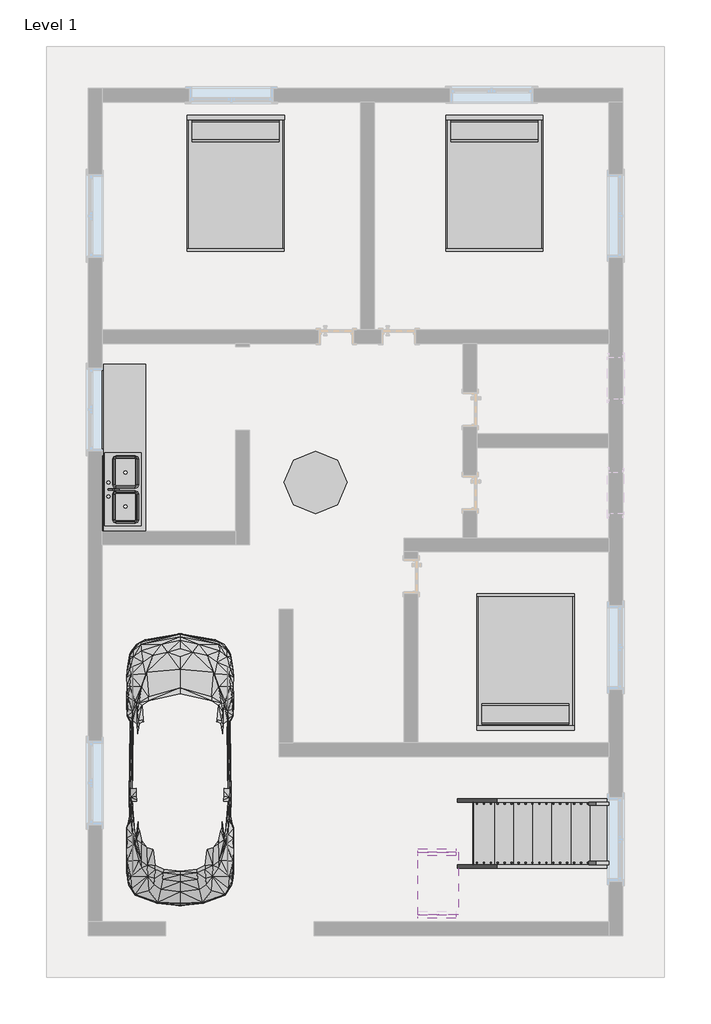
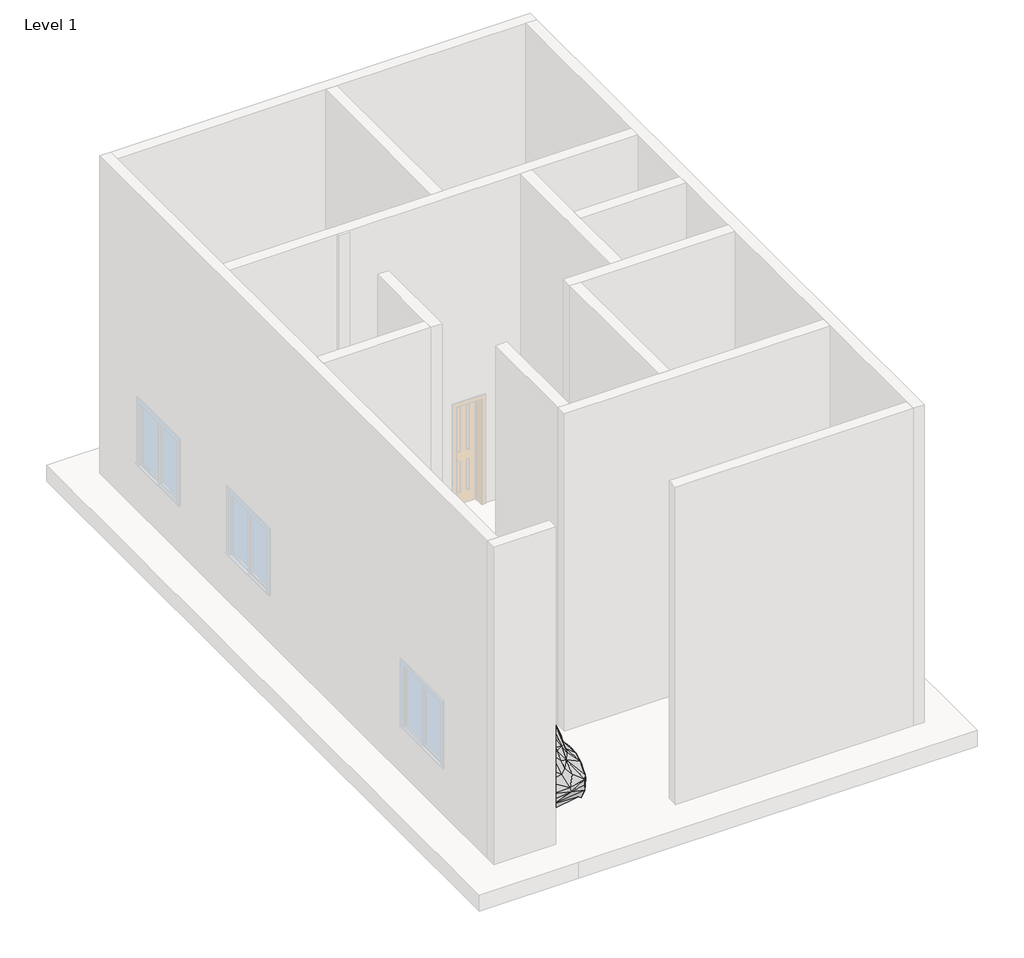
# One storey, part 2 of 2: 5 furniture elements, 4 members, 3 railings, 2 stair flights, 1 flow terminal, 1 proxy.
"""IFC4 building model written with IfcOpenShell, lengths in millimetres."""

from ifc_helpers import new_model, si_unit, frame, origin, place, context, project, spatial, polyline, outline, extrude, transform, mapped, element, save
from components import rpc_beetle_rpc_beetle_3ce7ba48, flow_terminal_a53be723, furniture_096e7f55, furniture_91b07d4a, furniture_905aceb5, stair_flight_75b00a3b, stair_flight_c315cc2a

model = new_model("IFC4")

# Units and contexts
model_context = context("Model", 3, world=origin())
ifc_project = project(units=[si_unit("LENGTHUNIT", "METRE", prefix="MILLI")], contexts=[model_context])

# Site, building, storey
site = spatial("IfcSite", under=ifc_project)
building = spatial("IfcBuilding", under=site)
storey = spatial("IfcBuildingStorey", under=building, Name="Level 1", Elevation=0.0)

# Proxy
placement = place(None, origin())
rpc_beetle_rpc_beetle_shape = rpc_beetle_rpc_beetle_3ce7ba48(model_context)
element("IfcBuildingElementProxy", 1, Name="RPC Beetle : RPC Beetle", ObjectType="RPC Beetle : RPC Beetle", at=placement, inside=storey, context=model_context, shape_type="MappedRepresentation", body=[
    mapped(rpc_beetle_rpc_beetle_shape, transform((-13294.6836698, -717.7093225, 0.0), x_axis=(1.0, 0.0, 0.0), y_axis=(0.0, 1.0, 0.0), z_axis=(0.0, 0.0, 1.0))),
])

# Flow terminal
flow_terminal_shape = flow_terminal_a53be723(model_context)
element("IfcFlowTerminal", 2, ObjectType="Sink Kitchen-Double : 42\" x 21\"", at=placement, inside=storey, context=model_context, shape_type="MappedRepresentation", body=[
    mapped(flow_terminal_shape, transform((-14130.5382687, 4600.601437, 0.0), x_axis=(0.0, 1.0, 0.0), y_axis=(-1.0, 0.0, 0.0), z_axis=(0.0, 0.0, 1.0))),
])

# Furniture
furniture_shape = furniture_096e7f55(model_context)
element("IfcFurniture", 3, ObjectType="Bed-Shaker : Double 56\" x 78\"", at=placement, inside=storey, context=model_context, shape_type="MappedRepresentation", body=[
    mapped(furniture_shape, transform((-12462.8336698, 10077.2906775, 0.0), x_axis=(1.0, 0.0, 0.0), y_axis=(0.0, 1.0, 0.0), z_axis=(0.0, 0.0, 1.0))),
])
element("IfcFurniture", 4, ObjectType="Bed-Shaker : Double 56\" x 78\"", at=placement, inside=storey, context=model_context, shape_type="MappedRepresentation", body=[
    mapped(furniture_shape, transform((-8678.2336698, 10077.2906775, 0.0), x_axis=(1.0, 0.0, 0.0), y_axis=(0.0, 1.0, 0.0), z_axis=(0.0, 0.0, 1.0))),
])
element("IfcFurniture", 5, ObjectType="Bed-Shaker : Double 56\" x 78\"", at=placement, inside=storey, context=model_context, shape_type="MappedRepresentation", body=[
    mapped(furniture_shape, transform((-8259.1336698, 1111.0906775, 0.0), x_axis=(-1.0, 0.0, 0.0), y_axis=(0.0, -1.0, 0.0), z_axis=(0.0, 0.0, 1.0))),
])
furniture_2_shape = furniture_91b07d4a(model_context)
element("IfcFurniture", 6, ObjectType="Counter Top w Sink : 24\" Depth", at=placement, inside=storey, context=model_context, shape_type="MappedRepresentation", body=[
    mapped(furniture_2_shape, transform((-14437.6836698, 5207.1529726, 0.0), x_axis=(0.0, 1.0, 0.0), y_axis=(-1.0, 0.0, 0.0), z_axis=(0.0, 0.0, 1.0))),
])
furniture_3_shape = furniture_905aceb5(model_context)
element("IfcFurniture", 7, ObjectType="Table-Dining Round w Chairs : 36\" Diameter", at=placement, inside=storey, context=model_context, shape_type="MappedRepresentation", body=[
    mapped(furniture_3_shape, transform((-11417.165637, 4902.769366, 0.0), x_axis=(1.0, 0.0, 0.0), y_axis=(0.0, 1.0, 0.0), z_axis=(0.0, 0.0, 1.0))),
])

# Members
element("IfcMember", 8, ObjectType="Stringer - 2\" Width", at=placement, inside=storey, context=model_context, shape_type="SweptSolid", body=[
    extrude(outline(polyline([(0.0, -7020.8836698), (212.114512, -7020.8836698), (2074.7811786, -10094.2836698), (1718.3724171, -10094.2836698), (0.0, -7258.9691815), (0.0, -7020.8836698)])), frame((0.0, -920.9093225, 0.0), z_axis=(0.0, 1.0, 0.0), x_axis=(0.0, 0.0, 1.0)), (0.0, 0.0, 1.0), 50.8),
])
element("IfcMember", 9, ObjectType="Stringer - 2\" Width", at=placement, inside=storey, context=model_context, shape_type="SweptSolid", body=[
    extrude(outline(polyline([(0.0, -7020.8836698), (212.114512, -7020.8836698), (2074.7811786, -10094.2836698), (1718.3724171, -10094.2836698), (0.0, -7258.9691815), (0.0, -7020.8836698)])), frame((0.0, 44.2906775, 0.0), z_axis=(0.0, 1.0, 0.0), x_axis=(0.0, 0.0, 1.0)), (0.0, 0.0, 1.0), 50.8),
])
element("IfcMember", 10, ObjectType="Stringer - 2\" Width", at=placement, inside=storey, context=model_context, shape_type="SweptSolid", body=[
    extrude(outline(polyline([(2244.114512, -9814.8836698), (1887.7057504, -9814.8836698), (2226.3724171, -9256.0836698), (2582.7811786, -9256.0836698), (2244.114512, -9814.8836698)])), frame((0.0, -692.3093225, 0.0), z_axis=(0.0, 1.0, 0.0), x_axis=(0.0, 0.0, 1.0)), (0.0, 0.0, 1.0), 50.8),
])
element("IfcMember", 11, ObjectType="Stringer - 2\" Width", at=placement, inside=storey, context=model_context, shape_type="SweptSolid", body=[
    extrude(outline(polyline([(2244.114512, -9814.8836698), (1887.7057504, -9814.8836698), (2226.3724171, -9256.0836698), (2582.7811786, -9256.0836698), (2244.114512, -9814.8836698)])), frame((0.0, -1657.5093225, 0.0), z_axis=(0.0, 1.0, 0.0), x_axis=(0.0, 0.0, 1.0)), (0.0, 0.0, 1.0), 50.8),
])

# Railings
element("IfcRailing", 12, ObjectType="Handrail - Rectangular", at=placement, inside=storey, context=model_context, shape_type="SweptSolid", body=[
    extrude(outline(polyline([(1024.3318731, -7020.8836698), (1083.7333333, -7020.8836698), (2946.4, -10094.2836698), (2886.9985397, -10094.2836698), (1024.3318731, -7020.8836698)])), frame((0.0, -6.5093225, 0.0), z_axis=(0.0, 1.0, 0.0), x_axis=(0.0, 0.0, 1.0)), (0.0, 0.0, 1.0), 50.8),
    extrude(outline(polyline([(2865.8318731, -10059.3586698), (2877.3773276, -10078.4086698), (1862.6666667, -10078.4086698), (1862.6666667, -10059.3586698), (2865.8318731, -10059.3586698)])), frame((0.0, 9.3656775, 0.0), z_axis=(0.0, 1.0, 0.0), x_axis=(0.0, 0.0, 1.0)), (0.0, 0.0, 1.0), 19.05),
    extrude(outline(polyline([(2804.2561155, -9957.7586698), (2815.80157, -9976.8086698), (1862.6666667, -9976.8086698), (1862.6666667, -9957.7586698), (2804.2561155, -9957.7586698)])), frame((0.0, 9.3656775, 0.0), z_axis=(0.0, 1.0, 0.0), x_axis=(0.0, 0.0, 1.0)), (0.0, 0.0, 1.0), 19.05),
    extrude(outline(polyline([(2742.6803579, -9856.1586698), (2754.2258125, -9875.2086698), (1862.6666667, -9875.2086698), (1862.6666667, -9856.1586698), (2742.6803579, -9856.1586698)])), frame((0.0, 9.3656775, 0.0), z_axis=(0.0, 1.0, 0.0), x_axis=(0.0, 0.0, 1.0)), (0.0, 0.0, 1.0), 19.05),
    extrude(outline(polyline([(2681.1046004, -9754.5586698), (2692.6500549, -9773.6086698), (1693.3333333, -9773.6086698), (1693.3333333, -9754.5586698), (2681.1046004, -9754.5586698)])), frame((0.0, 9.3656775, 0.0), z_axis=(0.0, 1.0, 0.0), x_axis=(0.0, 0.0, 1.0)), (0.0, 0.0, 1.0), 19.05),
    extrude(outline(polyline([(2619.5288428, -9652.9586698), (2631.0742973, -9672.0086698), (1693.3333333, -9672.0086698), (1693.3333333, -9652.9586698), (2619.5288428, -9652.9586698)])), frame((0.0, 9.3656775, 0.0), z_axis=(0.0, 1.0, 0.0), x_axis=(0.0, 0.0, 1.0)), (0.0, 0.0, 1.0), 19.05),
    extrude(outline(polyline([(2557.9530852, -9551.3586698), (2569.4985397, -9570.4086698), (1693.3333333, -9570.4086698), (1693.3333333, -9551.3586698), (2557.9530852, -9551.3586698)])), frame((0.0, 9.3656775, 0.0), z_axis=(0.0, 1.0, 0.0), x_axis=(0.0, 0.0, 1.0)), (0.0, 0.0, 1.0), 19.05),
    extrude(outline(polyline([(2496.3773276, -9449.7586698), (2507.9227822, -9468.8086698), (1524.0, -9468.8086698), (1524.0, -9449.7586698), (2496.3773276, -9449.7586698)])), frame((0.0, 9.3656775, 0.0), z_axis=(0.0, 1.0, 0.0), x_axis=(0.0, 0.0, 1.0)), (0.0, 0.0, 1.0), 19.05),
    extrude(outline(polyline([(2434.80157, -9348.1586698), (2446.3470246, -9367.2086698), (1524.0, -9367.2086698), (1524.0, -9348.1586698), (2434.80157, -9348.1586698)])), frame((0.0, 9.3656775, 0.0), z_axis=(0.0, 1.0, 0.0), x_axis=(0.0, 0.0, 1.0)), (0.0, 0.0, 1.0), 19.05),
    extrude(outline(polyline([(2373.2258125, -9246.5586698), (2384.771267, -9265.6086698), (1524.0, -9265.6086698), (1524.0, -9246.5586698), (2373.2258125, -9246.5586698)])), frame((0.0, 9.3656775, 0.0), z_axis=(0.0, 1.0, 0.0), x_axis=(0.0, 0.0, 1.0)), (0.0, 0.0, 1.0), 19.05),
    extrude(outline(polyline([(2311.6500549, -9144.9586698), (2323.1955094, -9164.0086698), (1354.6666667, -9164.0086698), (1354.6666667, -9144.9586698), (2311.6500549, -9144.9586698)])), frame((0.0, 9.3656775, 0.0), z_axis=(0.0, 1.0, 0.0), x_axis=(0.0, 0.0, 1.0)), (0.0, 0.0, 1.0), 19.05),
    extrude(outline(polyline([(2250.0742973, -9043.3586698), (2261.6197519, -9062.4086698), (1354.6666667, -9062.4086698), (1354.6666667, -9043.3586698), (2250.0742973, -9043.3586698)])), frame((0.0, 9.3656775, 0.0), z_axis=(0.0, 1.0, 0.0), x_axis=(0.0, 0.0, 1.0)), (0.0, 0.0, 1.0), 19.05),
    extrude(outline(polyline([(2188.4985397, -8941.7586698), (2200.0439943, -8960.8086698), (1185.3333333, -8960.8086698), (1185.3333333, -8941.7586698), (2188.4985397, -8941.7586698)])), frame((0.0, 9.3656775, 0.0), z_axis=(0.0, 1.0, 0.0), x_axis=(0.0, 0.0, 1.0)), (0.0, 0.0, 1.0), 19.05),
    extrude(outline(polyline([(2126.9227822, -8840.1586698), (2138.4682367, -8859.2086698), (1185.3333333, -8859.2086698), (1185.3333333, -8840.1586698), (2126.9227822, -8840.1586698)])), frame((0.0, 9.3656775, 0.0), z_axis=(0.0, 1.0, 0.0), x_axis=(0.0, 0.0, 1.0)), (0.0, 0.0, 1.0), 19.05),
    extrude(outline(polyline([(2065.3470246, -8738.5586698), (2076.8924791, -8757.6086698), (1185.3333333, -8757.6086698), (1185.3333333, -8738.5586698), (2065.3470246, -8738.5586698)])), frame((0.0, 9.3656775, 0.0), z_axis=(0.0, 1.0, 0.0), x_axis=(0.0, 0.0, 1.0)), (0.0, 0.0, 1.0), 19.05),
    extrude(outline(polyline([(2003.771267, -8636.9586698), (2015.3167216, -8656.0086698), (1016.0, -8656.0086698), (1016.0, -8636.9586698), (2003.771267, -8636.9586698)])), frame((0.0, 9.3656775, 0.0), z_axis=(0.0, 1.0, 0.0), x_axis=(0.0, 0.0, 1.0)), (0.0, 0.0, 1.0), 19.05),
    extrude(outline(polyline([(1942.1955094, -8535.3586698), (1953.740964, -8554.4086698), (1016.0, -8554.4086698), (1016.0, -8535.3586698), (1942.1955094, -8535.3586698)])), frame((0.0, 9.3656775, 0.0), z_axis=(0.0, 1.0, 0.0), x_axis=(0.0, 0.0, 1.0)), (0.0, 0.0, 1.0), 19.05),
    extrude(outline(polyline([(1880.6197519, -8433.7586698), (1892.1652064, -8452.8086698), (1016.0, -8452.8086698), (1016.0, -8433.7586698), (1880.6197519, -8433.7586698)])), frame((0.0, 9.3656775, 0.0), z_axis=(0.0, 1.0, 0.0), x_axis=(0.0, 0.0, 1.0)), (0.0, 0.0, 1.0), 19.05),
    extrude(outline(polyline([(1819.0439943, -8332.1586698), (1830.5894488, -8351.2086698), (846.6666667, -8351.2086698), (846.6666667, -8332.1586698), (1819.0439943, -8332.1586698)])), frame((0.0, 9.3656775, 0.0), z_axis=(0.0, 1.0, 0.0), x_axis=(0.0, 0.0, 1.0)), (0.0, 0.0, 1.0), 19.05),
    extrude(outline(polyline([(1757.4682367, -8230.5586698), (1769.0136913, -8249.6086698), (846.6666667, -8249.6086698), (846.6666667, -8230.5586698), (1757.4682367, -8230.5586698)])), frame((0.0, 9.3656775, 0.0), z_axis=(0.0, 1.0, 0.0), x_axis=(0.0, 0.0, 1.0)), (0.0, 0.0, 1.0), 19.05),
    extrude(outline(polyline([(1695.8924791, -8128.9586698), (1707.4379337, -8148.0086698), (846.6666667, -8148.0086698), (846.6666667, -8128.9586698), (1695.8924791, -8128.9586698)])), frame((0.0, 9.3656775, 0.0), z_axis=(0.0, 1.0, 0.0), x_axis=(0.0, 0.0, 1.0)), (0.0, 0.0, 1.0), 19.05),
    extrude(outline(polyline([(1634.3167216, -8027.3586698), (1645.8621761, -8046.4086698), (677.3333333, -8046.4086698), (677.3333333, -8027.3586698), (1634.3167216, -8027.3586698)])), frame((0.0, 9.3656775, 0.0), z_axis=(0.0, 1.0, 0.0), x_axis=(0.0, 0.0, 1.0)), (0.0, 0.0, 1.0), 19.05),
    extrude(outline(polyline([(1572.740964, -7925.7586698), (1584.2864185, -7944.8086698), (677.3333333, -7944.8086698), (677.3333333, -7925.7586698), (1572.740964, -7925.7586698)])), frame((0.0, 9.3656775, 0.0), z_axis=(0.0, 1.0, 0.0), x_axis=(0.0, 0.0, 1.0)), (0.0, 0.0, 1.0), 19.05),
    extrude(outline(polyline([(1511.1652064, -7824.1586698), (1522.710661, -7843.2086698), (508.0, -7843.2086698), (508.0, -7824.1586698), (1511.1652064, -7824.1586698)])), frame((0.0, 9.3656775, 0.0), z_axis=(0.0, 1.0, 0.0), x_axis=(0.0, 0.0, 1.0)), (0.0, 0.0, 1.0), 19.05),
    extrude(outline(polyline([(1449.5894488, -7722.5586698), (1461.1349034, -7741.6086698), (508.0, -7741.6086698), (508.0, -7722.5586698), (1449.5894488, -7722.5586698)])), frame((0.0, 9.3656775, 0.0), z_axis=(0.0, 1.0, 0.0), x_axis=(0.0, 0.0, 1.0)), (0.0, 0.0, 1.0), 19.05),
    extrude(outline(polyline([(1388.0136913, -7620.9586698), (1399.5591458, -7640.0086698), (508.0, -7640.0086698), (508.0, -7620.9586698), (1388.0136913, -7620.9586698)])), frame((0.0, 9.3656775, 0.0), z_axis=(0.0, 1.0, 0.0), x_axis=(0.0, 0.0, 1.0)), (0.0, 0.0, 1.0), 19.05),
    extrude(outline(polyline([(1326.4379337, -7519.3586698), (1337.9833882, -7538.4086698), (338.6666667, -7538.4086698), (338.6666667, -7519.3586698), (1326.4379337, -7519.3586698)])), frame((0.0, 9.3656775, 0.0), z_axis=(0.0, 1.0, 0.0), x_axis=(0.0, 0.0, 1.0)), (0.0, 0.0, 1.0), 19.05),
    extrude(outline(polyline([(1264.8621761, -7417.7586698), (1276.4076307, -7436.8086698), (338.6666667, -7436.8086698), (338.6666667, -7417.7586698), (1264.8621761, -7417.7586698)])), frame((0.0, 9.3656775, 0.0), z_axis=(0.0, 1.0, 0.0), x_axis=(0.0, 0.0, 1.0)), (0.0, 0.0, 1.0), 19.05),
    extrude(outline(polyline([(1203.2864185, -7316.1586698), (1214.8318731, -7335.2086698), (338.6666667, -7335.2086698), (338.6666667, -7316.1586698), (1203.2864185, -7316.1586698)])), frame((0.0, 9.3656775, 0.0), z_axis=(0.0, 1.0, 0.0), x_axis=(0.0, 0.0, 1.0)), (0.0, 0.0, 1.0), 19.05),
    extrude(outline(polyline([(1141.710661, -7214.5586698), (1153.2561155, -7233.6086698), (169.3333333, -7233.6086698), (169.3333333, -7214.5586698), (1141.710661, -7214.5586698)])), frame((0.0, 9.3656775, 0.0), z_axis=(0.0, 1.0, 0.0), x_axis=(0.0, 0.0, 1.0)), (0.0, 0.0, 1.0), 19.05),
    extrude(outline(polyline([(1080.1349034, -7112.9586698), (1091.6803579, -7132.0086698), (169.3333333, -7132.0086698), (169.3333333, -7112.9586698), (1080.1349034, -7112.9586698)])), frame((0.0, 9.3656775, 0.0), z_axis=(0.0, 1.0, 0.0), x_axis=(0.0, 0.0, 1.0)), (0.0, 0.0, 1.0), 19.05),
    extrude(outline(polyline([(2875.4530852, -10075.2336698), (2886.9985397, -10094.2836698), (1862.6666667, -10094.2836698), (1862.6666667, -10075.2336698), (2875.4530852, -10075.2336698)])), frame((0.0, 9.3656775, 0.0), z_axis=(0.0, 1.0, 0.0), x_axis=(0.0, 0.0, 1.0)), (0.0, 0.0, 1.0), 19.05),
    extrude(outline(polyline([(1024.3318731, -7020.8836698), (1035.8773276, -7039.9336698), (169.3333333, -7039.9336698), (169.3333333, -7020.8836698), (1024.3318731, -7020.8836698)])), frame((0.0, 9.3656775, 0.0), z_axis=(0.0, 1.0, 0.0), x_axis=(0.0, 0.0, 1.0)), (0.0, 0.0, 1.0), 19.05),
])
element("IfcRailing", 13, ObjectType="Handrail - Rectangular", at=placement, inside=storey, context=model_context, shape_type="SweptSolid", body=[
    extrude(outline(polyline([(1024.3318731, -7020.8836698), (1083.7333333, -7020.8836698), (2946.4, -10094.2836698), (2886.9985397, -10094.2836698), (1024.3318731, -7020.8836698)])), frame((0.0, -870.1093225, 0.0), z_axis=(0.0, 1.0, 0.0), x_axis=(0.0, 0.0, 1.0)), (0.0, 0.0, 1.0), 50.8),
    extrude(outline(polyline([(2877.3773276, -10078.4086698), (1862.6666667, -10078.4086698), (1862.6666667, -10059.3586698), (2865.8318731, -10059.3586698), (2877.3773276, -10078.4086698)])), frame((0.0, -854.2343225, 0.0), z_axis=(0.0, 1.0, 0.0), x_axis=(0.0, 0.0, 1.0)), (0.0, 0.0, 1.0), 19.05),
    extrude(outline(polyline([(2815.80157, -9976.8086698), (1862.6666667, -9976.8086698), (1862.6666667, -9957.7586698), (2804.2561155, -9957.7586698), (2815.80157, -9976.8086698)])), frame((0.0, -854.2343225, 0.0), z_axis=(0.0, 1.0, 0.0), x_axis=(0.0, 0.0, 1.0)), (0.0, 0.0, 1.0), 19.05),
    extrude(outline(polyline([(2754.2258125, -9875.2086698), (1862.6666667, -9875.2086698), (1862.6666667, -9856.1586698), (2742.6803579, -9856.1586698), (2754.2258125, -9875.2086698)])), frame((0.0, -854.2343225, 0.0), z_axis=(0.0, 1.0, 0.0), x_axis=(0.0, 0.0, 1.0)), (0.0, 0.0, 1.0), 19.05),
    extrude(outline(polyline([(2692.6500549, -9773.6086698), (2201.3333333, -9773.6086698), (2201.3333333, -9754.5586698), (2681.1046004, -9754.5586698), (2692.6500549, -9773.6086698)])), frame((0.0, -854.2343225, 0.0), z_axis=(0.0, 1.0, 0.0), x_axis=(0.0, 0.0, 1.0)), (0.0, 0.0, 1.0), 19.05),
    extrude(outline(polyline([(2631.0742973, -9672.0086698), (2201.3333333, -9672.0086698), (2201.3333333, -9652.9586698), (2619.5288428, -9652.9586698), (2631.0742973, -9672.0086698)])), frame((0.0, -854.2343225, 0.0), z_axis=(0.0, 1.0, 0.0), x_axis=(0.0, 0.0, 1.0)), (0.0, 0.0, 1.0), 19.05),
    extrude(outline(polyline([(2569.4985397, -9570.4086698), (2201.3333333, -9570.4086698), (2201.3333333, -9551.3586698), (2557.9530852, -9551.3586698), (2569.4985397, -9570.4086698)])), frame((0.0, -854.2343225, 0.0), z_axis=(0.0, 1.0, 0.0), x_axis=(0.0, 0.0, 1.0)), (0.0, 0.0, 1.0), 19.05),
    extrude(outline(polyline([(2507.9227822, -9468.8086698), (2370.6666667, -9468.8086698), (2370.6666667, -9449.7586698), (2496.3773276, -9449.7586698), (2507.9227822, -9468.8086698)])), frame((0.0, -854.2343225, 0.0), z_axis=(0.0, 1.0, 0.0), x_axis=(0.0, 0.0, 1.0)), (0.0, 0.0, 1.0), 19.05),
    extrude(outline(polyline([(2446.3470246, -9367.2086698), (2370.6666667, -9367.2086698), (2370.6666667, -9348.1586698), (2434.80157, -9348.1586698), (2446.3470246, -9367.2086698)])), frame((0.0, -854.2343225, 0.0), z_axis=(0.0, 1.0, 0.0), x_axis=(0.0, 0.0, 1.0)), (0.0, 0.0, 1.0), 19.05),
    extrude(outline(polyline([(2384.771267, -9265.6086698), (2370.6666667, -9265.6086698), (2370.6666667, -9246.5586698), (2373.2258125, -9246.5586698), (2384.771267, -9265.6086698)])), frame((0.0, -854.2343225, 0.0), z_axis=(0.0, 1.0, 0.0), x_axis=(0.0, 0.0, 1.0)), (0.0, 0.0, 1.0), 19.05),
    extrude(outline(polyline([(2323.1955094, -9164.0086698), (1354.6666667, -9164.0086698), (1354.6666667, -9144.9586698), (2311.6500549, -9144.9586698), (2323.1955094, -9164.0086698)])), frame((0.0, -854.2343225, 0.0), z_axis=(0.0, 1.0, 0.0), x_axis=(0.0, 0.0, 1.0)), (0.0, 0.0, 1.0), 19.05),
    extrude(outline(polyline([(2261.6197519, -9062.4086698), (1354.6666667, -9062.4086698), (1354.6666667, -9043.3586698), (2250.0742973, -9043.3586698), (2261.6197519, -9062.4086698)])), frame((0.0, -854.2343225, 0.0), z_axis=(0.0, 1.0, 0.0), x_axis=(0.0, 0.0, 1.0)), (0.0, 0.0, 1.0), 19.05),
    extrude(outline(polyline([(2200.0439943, -8960.8086698), (1185.3333333, -8960.8086698), (1185.3333333, -8941.7586698), (2188.4985397, -8941.7586698), (2200.0439943, -8960.8086698)])), frame((0.0, -854.2343225, 0.0), z_axis=(0.0, 1.0, 0.0), x_axis=(0.0, 0.0, 1.0)), (0.0, 0.0, 1.0), 19.05),
    extrude(outline(polyline([(2138.4682367, -8859.2086698), (1185.3333333, -8859.2086698), (1185.3333333, -8840.1586698), (2126.9227822, -8840.1586698), (2138.4682367, -8859.2086698)])), frame((0.0, -854.2343225, 0.0), z_axis=(0.0, 1.0, 0.0), x_axis=(0.0, 0.0, 1.0)), (0.0, 0.0, 1.0), 19.05),
    extrude(outline(polyline([(2076.8924791, -8757.6086698), (1185.3333333, -8757.6086698), (1185.3333333, -8738.5586698), (2065.3470246, -8738.5586698), (2076.8924791, -8757.6086698)])), frame((0.0, -854.2343225, 0.0), z_axis=(0.0, 1.0, 0.0), x_axis=(0.0, 0.0, 1.0)), (0.0, 0.0, 1.0), 19.05),
    extrude(outline(polyline([(2015.3167216, -8656.0086698), (1016.0, -8656.0086698), (1016.0, -8636.9586698), (2003.771267, -8636.9586698), (2015.3167216, -8656.0086698)])), frame((0.0, -854.2343225, 0.0), z_axis=(0.0, 1.0, 0.0), x_axis=(0.0, 0.0, 1.0)), (0.0, 0.0, 1.0), 19.05),
    extrude(outline(polyline([(1953.740964, -8554.4086698), (1016.0, -8554.4086698), (1016.0, -8535.3586698), (1942.1955094, -8535.3586698), (1953.740964, -8554.4086698)])), frame((0.0, -854.2343225, 0.0), z_axis=(0.0, 1.0, 0.0), x_axis=(0.0, 0.0, 1.0)), (0.0, 0.0, 1.0), 19.05),
    extrude(outline(polyline([(1892.1652064, -8452.8086698), (1016.0, -8452.8086698), (1016.0, -8433.7586698), (1880.6197519, -8433.7586698), (1892.1652064, -8452.8086698)])), frame((0.0, -854.2343225, 0.0), z_axis=(0.0, 1.0, 0.0), x_axis=(0.0, 0.0, 1.0)), (0.0, 0.0, 1.0), 19.05),
    extrude(outline(polyline([(1830.5894488, -8351.2086698), (846.6666667, -8351.2086698), (846.6666667, -8332.1586698), (1819.0439943, -8332.1586698), (1830.5894488, -8351.2086698)])), frame((0.0, -854.2343225, 0.0), z_axis=(0.0, 1.0, 0.0), x_axis=(0.0, 0.0, 1.0)), (0.0, 0.0, 1.0), 19.05),
    extrude(outline(polyline([(1769.0136913, -8249.6086698), (846.6666667, -8249.6086698), (846.6666667, -8230.5586698), (1757.4682367, -8230.5586698), (1769.0136913, -8249.6086698)])), frame((0.0, -854.2343225, 0.0), z_axis=(0.0, 1.0, 0.0), x_axis=(0.0, 0.0, 1.0)), (0.0, 0.0, 1.0), 19.05),
    extrude(outline(polyline([(1707.4379337, -8148.0086698), (846.6666667, -8148.0086698), (846.6666667, -8128.9586698), (1695.8924791, -8128.9586698), (1707.4379337, -8148.0086698)])), frame((0.0, -854.2343225, 0.0), z_axis=(0.0, 1.0, 0.0), x_axis=(0.0, 0.0, 1.0)), (0.0, 0.0, 1.0), 19.05),
    extrude(outline(polyline([(1645.8621761, -8046.4086698), (677.3333333, -8046.4086698), (677.3333333, -8027.3586698), (1634.3167216, -8027.3586698), (1645.8621761, -8046.4086698)])), frame((0.0, -854.2343225, 0.0), z_axis=(0.0, 1.0, 0.0), x_axis=(0.0, 0.0, 1.0)), (0.0, 0.0, 1.0), 19.05),
    extrude(outline(polyline([(1584.2864185, -7944.8086698), (677.3333333, -7944.8086698), (677.3333333, -7925.7586698), (1572.740964, -7925.7586698), (1584.2864185, -7944.8086698)])), frame((0.0, -854.2343225, 0.0), z_axis=(0.0, 1.0, 0.0), x_axis=(0.0, 0.0, 1.0)), (0.0, 0.0, 1.0), 19.05),
    extrude(outline(polyline([(1522.710661, -7843.2086698), (508.0, -7843.2086698), (508.0, -7824.1586698), (1511.1652064, -7824.1586698), (1522.710661, -7843.2086698)])), frame((0.0, -854.2343225, 0.0), z_axis=(0.0, 1.0, 0.0), x_axis=(0.0, 0.0, 1.0)), (0.0, 0.0, 1.0), 19.05),
    extrude(outline(polyline([(1461.1349034, -7741.6086698), (508.0, -7741.6086698), (508.0, -7722.5586698), (1449.5894488, -7722.5586698), (1461.1349034, -7741.6086698)])), frame((0.0, -854.2343225, 0.0), z_axis=(0.0, 1.0, 0.0), x_axis=(0.0, 0.0, 1.0)), (0.0, 0.0, 1.0), 19.05),
    extrude(outline(polyline([(1399.5591458, -7640.0086698), (508.0, -7640.0086698), (508.0, -7620.9586698), (1388.0136913, -7620.9586698), (1399.5591458, -7640.0086698)])), frame((0.0, -854.2343225, 0.0), z_axis=(0.0, 1.0, 0.0), x_axis=(0.0, 0.0, 1.0)), (0.0, 0.0, 1.0), 19.05),
    extrude(outline(polyline([(1337.9833882, -7538.4086698), (338.6666667, -7538.4086698), (338.6666667, -7519.3586698), (1326.4379337, -7519.3586698), (1337.9833882, -7538.4086698)])), frame((0.0, -854.2343225, 0.0), z_axis=(0.0, 1.0, 0.0), x_axis=(0.0, 0.0, 1.0)), (0.0, 0.0, 1.0), 19.05),
    extrude(outline(polyline([(1276.4076307, -7436.8086698), (338.6666667, -7436.8086698), (338.6666667, -7417.7586698), (1264.8621761, -7417.7586698), (1276.4076307, -7436.8086698)])), frame((0.0, -854.2343225, 0.0), z_axis=(0.0, 1.0, 0.0), x_axis=(0.0, 0.0, 1.0)), (0.0, 0.0, 1.0), 19.05),
    extrude(outline(polyline([(1214.8318731, -7335.2086698), (338.6666667, -7335.2086698), (338.6666667, -7316.1586698), (1203.2864185, -7316.1586698), (1214.8318731, -7335.2086698)])), frame((0.0, -854.2343225, 0.0), z_axis=(0.0, 1.0, 0.0), x_axis=(0.0, 0.0, 1.0)), (0.0, 0.0, 1.0), 19.05),
    extrude(outline(polyline([(1153.2561155, -7233.6086698), (169.3333333, -7233.6086698), (169.3333333, -7214.5586698), (1141.710661, -7214.5586698), (1153.2561155, -7233.6086698)])), frame((0.0, -854.2343225, 0.0), z_axis=(0.0, 1.0, 0.0), x_axis=(0.0, 0.0, 1.0)), (0.0, 0.0, 1.0), 19.05),
    extrude(outline(polyline([(1091.6803579, -7132.0086698), (169.3333333, -7132.0086698), (169.3333333, -7112.9586698), (1080.1349034, -7112.9586698), (1091.6803579, -7132.0086698)])), frame((0.0, -854.2343225, 0.0), z_axis=(0.0, 1.0, 0.0), x_axis=(0.0, 0.0, 1.0)), (0.0, 0.0, 1.0), 19.05),
    extrude(outline(polyline([(2886.9985397, -10094.2836698), (1862.6666667, -10094.2836698), (1862.6666667, -10075.2336698), (2875.4530852, -10075.2336698), (2886.9985397, -10094.2836698)])), frame((0.0, -854.2343225, 0.0), z_axis=(0.0, 1.0, 0.0), x_axis=(0.0, 0.0, 1.0)), (0.0, 0.0, 1.0), 19.05),
    extrude(outline(polyline([(1035.8773276, -7039.9336698), (169.3333333, -7039.9336698), (169.3333333, -7020.8836698), (1024.3318731, -7020.8836698), (1035.8773276, -7039.9336698)])), frame((0.0, -854.2343225, 0.0), z_axis=(0.0, 1.0, 0.0), x_axis=(0.0, 0.0, 1.0)), (0.0, 0.0, 1.0), 19.05),
])
element("IfcRailing", 14, ObjectType="Handrail - Rectangular", at=placement, inside=storey, context=model_context, shape_type="SweptSolid", body=[
    extrude(outline(polyline([(3115.7333333, -9814.8836698), (3056.3318731, -9814.8836698), (3394.9985397, -9256.0836698), (3454.4, -9256.0836698), (3115.7333333, -9814.8836698)])), frame((0.0, -743.1093225, 0.0), z_axis=(0.0, 1.0, 0.0), x_axis=(0.0, 0.0, 1.0)), (0.0, 0.0, 1.0), 50.8),
    extrude(outline(polyline([(3092.8924791, -9754.5586698), (3081.3470246, -9773.6086698), (2201.3333333, -9773.6086698), (2201.3333333, -9754.5586698), (3092.8924791, -9754.5586698)])), frame((0.0, -727.2343225, 0.0), z_axis=(0.0, 1.0, 0.0), x_axis=(0.0, 0.0, 1.0)), (0.0, 0.0, 1.0), 19.05),
    extrude(outline(polyline([(3154.4682367, -9652.9586698), (3142.9227822, -9672.0086698), (2201.3333333, -9672.0086698), (2201.3333333, -9652.9586698), (3154.4682367, -9652.9586698)])), frame((0.0, -727.2343225, 0.0), z_axis=(0.0, 1.0, 0.0), x_axis=(0.0, 0.0, 1.0)), (0.0, 0.0, 1.0), 19.05),
    extrude(outline(polyline([(3216.0439943, -9551.3586698), (3204.4985397, -9570.4086698), (2201.3333333, -9570.4086698), (2201.3333333, -9551.3586698), (3216.0439943, -9551.3586698)])), frame((0.0, -727.2343225, 0.0), z_axis=(0.0, 1.0, 0.0), x_axis=(0.0, 0.0, 1.0)), (0.0, 0.0, 1.0), 19.05),
    extrude(outline(polyline([(3277.6197519, -9449.7586698), (3266.0742973, -9468.8086698), (2370.6666667, -9468.8086698), (2370.6666667, -9449.7586698), (3277.6197519, -9449.7586698)])), frame((0.0, -727.2343225, 0.0), z_axis=(0.0, 1.0, 0.0), x_axis=(0.0, 0.0, 1.0)), (0.0, 0.0, 1.0), 19.05),
    extrude(outline(polyline([(3339.1955094, -9348.1586698), (3327.6500549, -9367.2086698), (2370.6666667, -9367.2086698), (2370.6666667, -9348.1586698), (3339.1955094, -9348.1586698)])), frame((0.0, -727.2343225, 0.0), z_axis=(0.0, 1.0, 0.0), x_axis=(0.0, 0.0, 1.0)), (0.0, 0.0, 1.0), 19.05),
    extrude(outline(polyline([(3067.8773276, -9795.8336698), (3056.3318731, -9814.8836698), (2201.3333333, -9814.8836698), (2201.3333333, -9795.8336698), (3067.8773276, -9795.8336698)])), frame((0.0, -727.2343225, 0.0), z_axis=(0.0, 1.0, 0.0), x_axis=(0.0, 0.0, 1.0)), (0.0, 0.0, 1.0), 19.05),
    extrude(outline(polyline([(3394.9985397, -9256.0836698), (3383.4530852, -9275.1336698), (2370.6666667, -9275.1336698), (2370.6666667, -9256.0836698), (3394.9985397, -9256.0836698)])), frame((0.0, -727.2343225, 0.0), z_axis=(0.0, 1.0, 0.0), x_axis=(0.0, 0.0, 1.0)), (0.0, 0.0, 1.0), 19.05),
])

# Stair flights
stair_flight_shape = stair_flight_75b00a3b(model_context)
element("IfcStairFlight", 15, ObjectType="2\" Tread 1\" Nosing 1/4\" Riser", at=placement, inside=storey, context=model_context, shape_type="MappedRepresentation", body=[
    mapped(stair_flight_shape, transform((0.0, 0.0, 0.0), x_axis=(1.0, 0.0, 0.0), y_axis=(0.0, 1.0, 0.0), z_axis=(0.0, 0.0, 1.0))),
])
stair_flight_2_shape = stair_flight_c315cc2a(model_context)
element("IfcStairFlight", 16, ObjectType="2\" Tread 1\" Nosing 1/4\" Riser", at=placement, inside=storey, context=model_context, shape_type="MappedRepresentation", body=[
    mapped(stair_flight_2_shape, transform((0.0, 0.0, 0.0), x_axis=(1.0, 0.0, 0.0), y_axis=(0.0, 1.0, 0.0), z_axis=(0.0, 0.0, 1.0))),
])

save(model, "model.ifc")

# Revit data of these elements
# Type "RPC Beetle : RPC Beetle"
#   built-in parameter 1005195 = "RPC-16-0U6E-L4EG-ENH1-J3KF-SVEL-0TX4-C0"
#   Height = 0
# Type "Sink Kitchen-Double : 42\" x 21\""
#   Assembly Code = "D2010410"
#   Counter Height = 3' - 0"
#   Depth = 1' - 9"
#   Width = 3' - 6"
#   Faucet Material = Steel, Polished
#   Sink Material = Steel, Polished
#   Default Elevation = 0
# Type "Bed-Shaker : Double 56\" x 78\""
#   Assembly Code = "E2020200"
#   Length = 6' - 6"
#   Width = 4' - 8"
#   Frame Material = Birch
#   Mattress Material = Linen, White
#   Default Elevation = 0
# Type "Counter Top w Sink : 24\" Depth"
#   Assembly Code = "C1030400"
#   Counter Thickness = 0' - 1 1/2"
#   Depth = 2' - 1"
#   Height = 3' - 0"
#   Length [instance default] = 8' - 0"
#   Sink Location [instance default] = 2' - 0"
#   Sink Location To Wall [instance default] = 0' - 6"
#   Sink Opening Depth [instance default] = 1' - 3"
#   Sink Opening Width [instance default] = 3' - 3"
#   Counter Top Material = none
#   Default Elevation = 0
# Type "Table-Dining Round w Chairs : 36\" Diameter"
#   Assembly Code = "E2020200"
#   Radius = 1' - 6"
#   Diameter = 3' - 0"
#   Height = 2' - 6"
#   Chairs = 4
#   Base Material = Pine
#   Top Material = Laminate, Linen, Matte
#   Default Elevation = 0
# Type "Handrail - Rectangular"
#   Assembly Code = "C2010400"
#   built-in parameter 1008612 = 0.0416667 (stored number, unit not read)
#   built-in parameter 1008611 = 0.0416667 (stored number, unit not read)
#   built-in parameter 1008609 = 0.333333 (stored number, unit not read)
#   built-in parameter 1008604 = 0.166667 (stored number, unit not read)
#   built-in parameter 1008603 = 0.166667 (stored number, unit not read)
#   Railing Height = 3' - 0"
#   built-in parameter 1008630 = 2
#   built-in parameter 1008610 = 2
#   built-in parameter 1008618 = Baluster - Square : 3/4"
# Element 1 (IfcBuildingElementProxy, "RPC Beetle : RPC Beetle")
#   Phase Created = New Construction
# Element 2 (IfcFlowTerminal, "Sink Kitchen-Double : 42\" x 21\"")
#   Mark = "1"
#   Phase Created = New Construction
#   Materials on its faces: "Steel, Polished"
# Elements 3, 4, 5 (IfcFurniture, "Bed-Shaker : Double 56\" x 78\"")
#   Phase Created = New Construction
#   Materials on its faces: "Birch", "Linen, White"
# Element 6 (IfcFurniture, "Counter Top w Sink : 24\" Depth")
#   Sink Opening Width = 3' - 3"
#   Sink Opening Depth = 1' - 3"
#   Sink Location To Wall = 0' - 6"
#   Sink Location = 2' - 0"
#   Length = 8' - 0"
#   Phase Created = New Construction
#   Materials on its faces: "Counter Top"
# Element 7 (IfcFurniture, "Table-Dining Round w Chairs : 36\" Diameter")
#   Phase Created = New Construction
#   Materials on its faces: "Pine", "Laminate, Linen, Matte"
# Elements 8, 9, 10, 11 (IfcMember, "Stringer - 2\" Width")
#   Phase Created = New Construction
# Elements 12, 13, 14 (IfcRailing, "Handrail - Rectangular")
#   Phase Created = New Construction
# Elements 15, 16 (IfcStairFlight, "2\" Tread 1\" Nosing 1/4\" Riser")
#   Phase Created = New Construction
# Materials
#   "Steel, Polished": class "Metal", colour RGB 192 192 192, transparency 0, Description = "Polished steel", Cost = 0
#   "Birch": class "Wood", colour RGB 224 178 126, transparency 0, Description = "Betula Alleghaniensis", Cost = 0
#   "Linen, White": class "Textile", colour RGB 247 247 239, transparency 0, Description = "Linen, white", Cost = 0
#   "Pine": class "Wood", colour RGB 223 192 134, transparency 0, Description = "Pinus Echinata", Cost = 0
#   "Laminate, Linen, Matte": class "Plastic", colour RGB 249 239 230, transparency 0, Description = "Plastic Laminate - Linen, Matte", Cost = 0
#   "Counter Top": class "Wood", colour RGB 226 177 128, transparency 0
